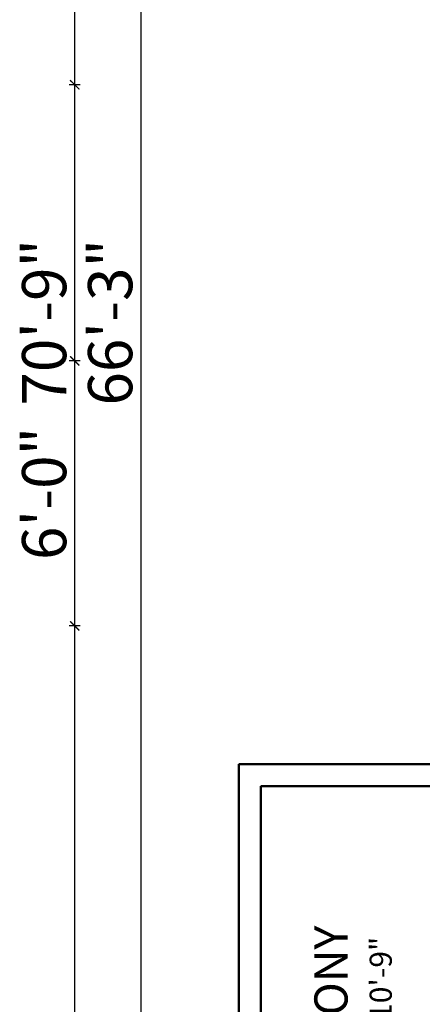
# Model space of a CAD drawing. Units: inches. Extents: x 375 to 1122, y 27 to 1069.
# Tile 68 of 155: x 385 to 494, y 400 to 667. Entities that reach past the tile are written whole.
import ezdxf

# ---------------------------------------------------------------- set-up
doc = ezdxf.new("R2010")
doc.units = ezdxf.units.IN
for name, color, linetype, lineweight in [('A-ANNO-DIMS', 2, 'Continuous', 18), ('A-AREA-IDEN', 7, 'Continuous', 18), ('Walls', 250, 'Continuous', 50)]:
    doc.layers.add(name, color=color, linetype=linetype, lineweight=lineweight)
doc.styles.get("Standard").update_dxf_attribs({"font": 'arial.ttf'})
doc.dimstyles.new('ISO-25', dxfattribs={"dimtxt": 12, "dimasz": 2.5, "dimexe": 1.5, "dimexo": 1.5, "dimtad": 1, "dimdec": 1, "dimlunit": 3, "dimtxsty": 'Standard', "dimblk": 'ARCHTICK', "dimcen": 2.5, "dimadec": 0, "dimazin": 0, "dimtfac": 1, "dimtdec": 1, "dimtmove": 0, "dimatfit": 3, "dimfxl": 1.5, "dimfxlon": 1, "dimarcsym": 0})

# ---------------------------------------------------------------- blocks, each defined once
blk = doc.blocks.new('_ArchTick')
at = {"color": 0, "linetype": 'ByBlock', "const_width": 0.15}
blk.add_lwpolyline([(-0.5, -0.5), (0.5, 0.5)], dxfattribs=at)
blk = doc.blocks.new('*D28')
at = {"layer": 'A-ANNO-DIMS', "color": 0, "lineweight": -2, "transparency": 16777216}
for p, q in [((419.42, 982.53), (416.42, 982.53)), ((417.92, 982.53), (417.92, 187.53)), ((419.42, 187.53), (416.42, 187.53))]:
    blk.add_line(p, q, dxfattribs=at)
at = {"layer": 'Defpoints', "color": 0, "transparency": 16777216}
for p in [(444.51, 982.53), (417.92, 187.53), (444.51, 187.53)]:
    blk.add_point(p, dxfattribs=at)
at = {"layer": 'A-ANNO-DIMS', "color": 0, "lineweight": -2, "transparency": 16777216, "xscale": 2.5, "yscale": 2.5, "zscale": 2.5}
for p, rotation in [((417.92, 982.53), 90), ((417.92, 187.53), 270)]:
    blk.add_blockref('_ArchTick', p, dxfattribs=dict(at, rotation=rotation))
at = {"layer": 'A-ANNO-DIMS', "color": 0, "transparency": 16777216, "insert": (411.17, 585.03), "char_height": 12, "attachment_point": 5, "rotation": 90}
blk.add_mtext('66\'-3"', dxfattribs=at)
blk = doc.blocks.new('*D69')
at = {"layer": 'A-ANNO-DIMS', "color": 0, "lineweight": -2, "transparency": 16777216}
for p, q in [((518.31, 685.53), (518.31, 841.13)), ((516.81, 685.53), (519.81, 685.53)), ((518.31, 613.53), (518.31, 685.53)), ((516.81, 613.53), (519.81, 613.53))]:
    blk.add_line(p, q, dxfattribs=at)
at = {"layer": 'Defpoints', "color": 0, "transparency": 16777216}
for p in [(507.51, 685.53), (518.31, 685.53), (507.51, 613.53)]:
    blk.add_point(p, dxfattribs=at)
at = {"layer": 'A-ANNO-DIMS', "color": 0, "lineweight": -2, "transparency": 16777216, "xscale": 2.5, "yscale": 2.5, "zscale": 2.5}
for p, rotation in [((518.31, 685.53), 90), ((518.31, 613.53), 270)]:
    blk.add_blockref('_ArchTick', p, dxfattribs=dict(at, rotation=rotation))
at = {"layer": 'A-ANNO-DIMS', "color": 0, "transparency": 16777216, "insert": (511.47, 764.58), "char_height": 12, "attachment_point": 5, "rotation": 90}
blk.add_mtext('WINDOW 6\'-0" TYP.', dxfattribs=at)
blk = doc.blocks.new('*D71')
at = {"layer": 'A-ANNO-DIMS', "color": 0, "lineweight": -2, "transparency": 16777216}
for p, q in [((520.11, 444.53), (520.11, 661.17)), ((518.61, 444.53), (521.61, 444.53)), ((520.11, 360.53), (520.11, 444.53)), ((518.61, 360.53), (521.61, 360.53))]:
    blk.add_line(p, q, dxfattribs=at)
at = {"layer": 'Defpoints', "color": 0, "transparency": 16777216}
for p in [(507.51, 444.53), (520.11, 444.53), (507.51, 360.53)]:
    blk.add_point(p, dxfattribs=at)
at = {"layer": 'A-ANNO-DIMS', "color": 0, "lineweight": -2, "transparency": 16777216, "xscale": 2.5, "yscale": 2.5, "zscale": 2.5}
for p, rotation in [((520.11, 444.53), 90), ((520.11, 360.53), 270)]:
    blk.add_blockref('_ArchTick', p, dxfattribs=dict(at, rotation=rotation))
at = {"layer": 'A-ANNO-DIMS', "color": 0, "transparency": 16777216, "insert": (513.27, 554.1), "char_height": 12, "attachment_point": 5, "rotation": 90}
blk.add_mtext('3-PANEL SLIDER 7\'-0" TYP.', dxfattribs=at)
blk = doc.blocks.new('*D82')
at = {"layer": 'A-ANNO-DIMS', "color": 0, "lineweight": -2, "transparency": 16777216}
for p, q in [((401.51, 1009.53), (398.51, 1009.53)), ((400.01, 160.53), (400.01, 1009.53)), ((401.51, 160.53), (398.51, 160.53))]:
    blk.add_line(p, q, dxfattribs=at)
at = {"layer": 'Defpoints', "color": 0, "transparency": 16777216}
for p in [(400.01, 1009.53), (630.53, 1009.53), (630.53, 160.53)]:
    blk.add_point(p, dxfattribs=at)
at = {"layer": 'A-ANNO-DIMS', "color": 0, "lineweight": -2, "transparency": 16777216, "xscale": 2.5, "yscale": 2.5, "zscale": 2.5}
for p, rotation in [((400.01, 1009.53), 90), ((400.01, 160.53), 270)]:
    blk.add_blockref('_ArchTick', p, dxfattribs=dict(at, rotation=rotation))
at = {"layer": 'A-ANNO-DIMS', "color": 0, "transparency": 16777216, "insert": (393.26, 585.03), "char_height": 12, "attachment_point": 5, "rotation": 90}
blk.add_mtext('70\'-9"', dxfattribs=at)
blk = doc.blocks.new('*D90')
at = {"layer": 'A-ANNO-DIMS', "color": 0, "lineweight": -2, "transparency": 16777216}
for p, q in [((401.51, 574.53), (398.51, 574.53)), ((400.01, 502.53), (400.01, 574.53)), ((401.51, 502.53), (398.51, 502.53))]:
    blk.add_line(p, q, dxfattribs=at)
at = {"layer": 'Defpoints', "color": 0, "transparency": 16777216}
for p in [(400.01, 574.53), (863.01, 574.53), (863.01, 502.53)]:
    blk.add_point(p, dxfattribs=at)
at = {"layer": 'A-ANNO-DIMS', "color": 0, "lineweight": -2, "transparency": 16777216, "xscale": 2.5, "yscale": 2.5, "zscale": 2.5}
for p, rotation in [((400.01, 574.53), 90), ((400.01, 502.53), 270)]:
    blk.add_blockref('_ArchTick', p, dxfattribs=dict(at, rotation=rotation))
at = {"layer": 'A-ANNO-DIMS', "color": 0, "transparency": 16777216, "insert": (393.26, 538.53), "char_height": 12, "attachment_point": 5, "rotation": 90}
blk.add_mtext('6\'-0"', dxfattribs=at)
blk = doc.blocks.new('*D93')
at = {"layer": 'A-ANNO-DIMS', "color": 0, "lineweight": -2, "transparency": 16777216}
for p, q in [((400.01, 673.53), (400.01, 709.38)), ((401.51, 673.53), (398.51, 673.53)), ((400.01, 649.53), (400.01, 673.53)), ((401.51, 649.53), (398.51, 649.53))]:
    blk.add_line(p, q, dxfattribs=at)
at = {"layer": 'Defpoints', "color": 0, "transparency": 16777216}
for p in [(400.01, 673.53), (663.51, 673.53), (663.51, 649.53)]:
    blk.add_point(p, dxfattribs=at)
at = {"layer": 'A-ANNO-DIMS', "color": 0, "lineweight": -2, "transparency": 16777216, "xscale": 2.5, "yscale": 2.5, "zscale": 2.5}
for p, rotation in [((400.01, 673.53), 90), ((400.01, 649.53), 270)]:
    blk.add_blockref('_ArchTick', p, dxfattribs=dict(at, rotation=rotation))
at = {"layer": 'A-ANNO-DIMS', "color": 0, "transparency": 16777216, "insert": (393.26, 692.7), "char_height": 12, "attachment_point": 5, "rotation": 90}
blk.add_mtext('2\'-0"', dxfattribs=at)

msp = doc.modelspace()

# ---------------------------------------------------------------- linework, layer by layer
at = {"layer": 'Walls'}
for p, q in [((444.51, 324.03), (444.51, 465.03)), ((444.51, 465.03), (498.51, 465.03)), ((450.51, 330.03), (450.51, 459.03)), ((450.51, 459.03), (498.51, 459.03))]:
    msp.add_line(p, q, dxfattribs=at)

# ---------------------------------------------------------------- texts
at = {"layer": 'A-AREA-IDEN', "insert": (465.03, 360.85), "char_height": 12, "attachment_point": 1, "rotation": 90}
msp.add_mtext_dynamic_manual_height_columns('\\pxqc;{\\fArial|b1|i0|c0|p34;\\H0.75x;BALCONY\\H1.33333x;\\P\\fArial|b0|i0|c0|p34;\\H0.5x;4\'-0" x 10\'-9"}', width=66.1169, gutter_width=12.5, heights=[0], dxfattribs=at)

# ---------------------------------------------------------------- dimensions: what is measured, and where the dimension line sits
at = {"layer": 'A-ANNO-DIMS'}
for base, p1, p2, override, picture, middle in [((400.01, 1009.53), (630.53, 160.53), (630.53, 1009.53), {"dimdec": 1, "dimlfac": 1, "dimrnd": 0, "dimzin": 1, "dimdsep": 46, "dimlunit": 4, "dimfrac": 2}, '*D82', (393.26, 585.03)), ((417.92, 187.53), (444.51, 982.53), (444.51, 187.53), {"dimclrd": 0, "dimclre": 0, "dimclrt": 0}, '*D28', (411.17, 585.03)), ((400.01, 673.53), (663.51, 649.53), (663.51, 673.53), {"dimdec": 1, "dimlfac": 1, "dimrnd": 0, "dimzin": 1, "dimdsep": 46, "dimlunit": 4, "dimfrac": 2}, '*D93', (393.26, 692.7)), ((400.01, 574.53), (863.01, 502.53), (863.01, 574.53), {"dimdec": 1, "dimlfac": 1, "dimrnd": 0, "dimzin": 1, "dimdsep": 46, "dimlunit": 4, "dimfrac": 2}, '*D90', (393.26, 538.53))]:
    dim = msp.add_linear_dim(base=base, p1=p1, p2=p2, angle=90, dimstyle='ISO-25', override=override, dxfattribs=at)
    dim.commit()
    dim.dimension.update_dxf_attribs({"geometry": picture, "text_midpoint": middle})
for base, p1, p2, text, picture, middle in [((518.31, 685.53), (507.51, 613.53), (507.51, 685.53), 'WINDOW <> TYP.', '*D69', (511.47, 764.58)), ((520.11, 444.53), (507.51, 360.53), (507.51, 444.53), '3-PANEL SLIDER <> TYP.', '*D71', (513.27, 554.1))]:
    dim = msp.add_linear_dim(base=base, p1=p1, p2=p2, angle=90, text=text, dimstyle='ISO-25', override={"dimdec": 1, "dimlfac": 1, "dimrnd": 0, "dimzin": 1, "dimdsep": 46, "dimlunit": 4, "dimfrac": 2}, dxfattribs=at)
    dim.commit()
    dim.dimension.update_dxf_attribs({"geometry": picture, "text_midpoint": middle})

doc.saveas('drawing.dxf')
